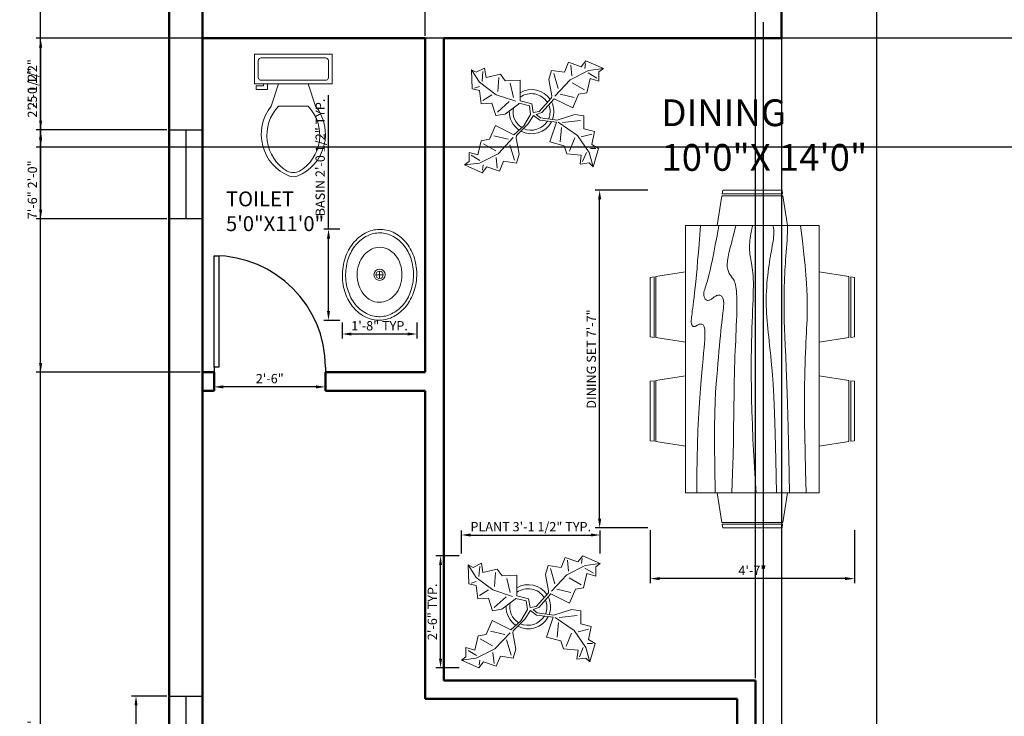
# Model space of a CAD drawing. Units: inches. Extents: x 25547 to 25983, y 30413 to 31159.
# Tile 3 of 5: x 25547 to 25813, y 30790 to 30978. Entities that reach past the tile are written whole.
import ezdxf

# ---------------------------------------------------------------- set-up
doc = ezdxf.new("R2010")
doc.units = ezdxf.units.IN
for name, color, linetype, lineweight in [('A-AREA-IDEN', 11, 'Continuous', 25), ('A-FLOR-FIXT', 6, 'Continuous', 18), ('A-WALL', 7, 'Continuous', 50), ('DIM', 4, 'Continuous', 18), ('DOOR', 3, 'Continuous', 25), ('FLOWER', 60, 'Continuous', 13), ('FURNITURES', 6, 'Continuous', 18), ('WINDOW', 1, 'Continuous', 25)]:
    doc.layers.add(name, color=color, linetype=linetype, lineweight=lineweight)
doc.styles.get("Standard").update_dxf_attribs({"font": 'arial.ttf'})
doc.dimstyles.new('ISO-25', dxfattribs={"dimtxt": 2.5, "dimasz": 2.5, "dimexe": 1.25, "dimexo": 0.625, "dimtad": 1, "dimlunit": 3, "dimtxsty": 'Standard', "dimcen": 2.5, "dimadec": 0, "dimazin": 0, "dimtfac": 1, "dimtmove": 0, "dimatfit": 3, "dimfxl": 1, "dimarcsym": 0})

# ---------------------------------------------------------------- blocks, each defined once
blk = doc.blocks.new('*U5')
for p, q in [((0, 0), (0, -6)), ((40, 0), (40, -6))]:
    blk.add_line(p, q)
blk.add_lwpolyline([(0, 0), (0, 40), (1.75, 40), (1.75, 0)], close=True)
blk.add_arc((0, 0), 40, 0, 90)
blk = doc.blocks.new('Sink - Oval top')
for p, q in [((-1, 0), (1, 0)), ((0, 1), (0, -1))]:
    blk.add_line(p, q)
for points in [[(-12.23, 0.39, 0.117634), (-11.46, -3.36, 0.104469), (-8.88, -6.8, 0.090016), (-5.08, -9.07, 0.08192), (-0.32, -10.02, 0.08192), (4.49, -9.38, 0.090016), (8.42, -7.36, 0.104469), (11.22, -4.09, 0.117634), (12.23, -0.39, 0.117634), (11.46, 3.36, 0.104469), (8.88, 6.8, 0.090016), (5.08, 9.07, 0.08192), (0.32, 10.02, 0.08192), (-4.49, 9.38, 0.090016), (-8.42, 7.36, 0.104469), (-11.22, 4.09, 0.117634)], [(-11.29, 0.16, 0.118622), (-10.52, -3.25, 0.104678), (-8.07, -6.36, 0.089562), (-4.54, -8.37, 0.081185), (-0.13, -9.15, 0.081185), (4.3, -8.49, 0.089562), (7.89, -6.58, 0.104678), (10.42, -3.55, 0.118622), (11.29, -0.16, 0.118622), (10.52, 3.25, 0.104678), (8.07, 6.36, 0.089562), (4.54, 8.37, 0.081185), (0.13, 9.15, 0.081185), (-4.3, 8.49, 0.089562), (-7.89, 6.58, 0.104678), (-10.42, 3.55, 0.118622)], [(-7.42, 0.08, 0.118283), (-6.91, -2.17, 0.104607), (-5.29, -4.21, 0.089718), (-2.97, -5.53, 0.081436), (-0.07, -6.04, 0.081436), (2.84, -5.59, 0.089718), (5.2, -4.33, 0.104607), (6.86, -2.32, 0.118283), (7.42, -0.08, 0.118283), (6.91, 2.17, 0.104607), (5.29, 4.21, 0.089718), (2.97, 5.53, 0.081436), (0.07, 6.04, 0.081436), (-2.84, 5.59, 0.089718), (-5.2, 4.33, 0.104607), (-6.86, 2.32, 0.118283)]]:
    blk.add_lwpolyline(points, format="xyb", close=True)
for radius in [1.5, 1]:
    blk.add_circle((0, 0), radius)
blk = doc.blocks.new('Dining Set - 36 x 72 in.')
for p, q in [((-22, 27.5), (-22.1562, 26.50042)), ((-22, 27.5), (-6, 27.5)), ((-5.8437, 26.49966), (-6, 27.5)), ((6, 27.5), (5.8438, 26.50042)), ((6, 27.5), (22, 27.5)), ((22.1563, 26.49966), (22, 27.5)), ((-22.2343, 26.00059), (-23.4847, 17.99762)), ((-22.2304, 26), (-5.7608, 26)), ((-5.8416, 26.5), (-22.1534, 26.5)), ((-4.5152, 17.99762), (-5.7655, 25.99926)), ((5.7657, 26.00059), (4.5153, 17.99762)), ((5.7696, 26), (22.2392, 26)), ((22.1584, 26.5), (5.8466, 26.5)), ((23.4848, 17.99762), (22.2345, 25.99926)), ((36, 18), (-36, 18)), ((-36, 18), (-36, -18)), ((36, -18), (36, 18)), ((-45.5, 8), (-44.5004, 8.15617)), ((-45.5, 8), (-45.5, -8)), ((-44.5, -8.15843), (-44.5, 8.15338)), ((-44.0006, 8.23428), (-35.9976, 9.48474)), ((-44, 8.23041), (-44, -8.23915)), ((44.0006, 8.23428), (35.9976, 9.48474)), ((44, 8.23041), (44, -8.23915)), ((44.5, -8.15843), (44.5, 8.15338)), ((45.5, 8), (44.5005, 8.15617)), ((45.5, 8), (45.5, -8)), ((-44.4997, -8.15631), (-45.5, -8)), ((-35.9976, -9.48476), (-43.9993, -8.2345)), ((35.9976, -9.48476), (43.9993, -8.2345)), ((44.4997, -8.15631), (45.5, -8)), ((-36, -18), (36, -18)), ((-22.2343, -26.0006), (-23.4847, -17.99762)), ((-4.5152, -17.99762), (-5.7655, -25.99928)), ((5.7657, -26.0006), (4.5153, -17.99762)), ((23.4848, -17.99762), (22.2345, -25.99928)), ((-22.2304, -26), (-5.7608, -26)), ((-22, -27.5), (-22.1562, -26.50044)), ((-5.8416, -26.5), (-22.1534, -26.5)), ((-5.8437, -26.49967), (-6, -27.5)), ((5.7696, -26), (22.2392, -26)), ((6, -27.5), (5.8438, -26.50044)), ((22.1584, -26.5), (5.8466, -26.5)), ((22.1563, -26.49967), (22, -27.5)), ((-22, -27.5), (-6, -27.5)), ((6, -27.5), (22, -27.5))]:
    blk.add_line(p, q)
for points in [[(-36, 15), (-31.1772, 14.97754), (-26.8079, 14.91406), (-22.8538, 14.81543), (-19.276, 14.6875), (-16.0362, 14.53613), (-13.0957, 14.36718), (-10.4159, 14.18652), (-7.9583, 14), (-5.6904, 13.81315), (-3.6035, 13.63021), (-1.6954, 13.45508), (0.0365, 13.29166), (1.5945, 13.14388), (2.9811, 13.01562), (4.1988, 12.9108), (5.25, 12.83333), (6.1393, 12.78613), (6.8802, 12.76823), (7.4883, 12.77767), (7.9792, 12.8125), (8.3685, 12.87077), (8.6719, 12.95052), (8.9049, 13.0498), (9.0833, 13.16666), (9.2205, 13.29899), (9.3216, 13.44401), (9.3895, 13.59879), (9.4271, 13.76041), (9.4373, 13.92594), (9.4232, 14.09245), (9.3875, 14.257), (9.3333, 14.41666), (9.2638, 14.56917), (9.1836, 14.71484), (9.0975, 14.85465), (9.0104, 14.98958), (8.9272, 15.1206), (8.8529, 15.2487), (8.7922, 15.37483), (8.75, 15.5), (8.7305, 15.62467), (8.7344, 15.74739), (8.7617, 15.86621), (8.8125, 15.97916), (8.8867, 16.08431), (8.9844, 16.17968), (9.1055, 16.26334), (9.25, 16.33333), (9.4189, 16.38802), (9.6172, 16.42708), (9.8506, 16.45052), (10.125, 16.45833), (10.4463, 16.45052), (10.8203, 16.42708), (11.2529, 16.38802), (11.75, 16.33333), (12.3184, 16.26318), (12.9694, 16.17838), (13.7151, 16.07991), (14.5677, 15.96875), (15.5395, 15.84586), (16.6426, 15.71224), (17.8893, 15.56884), (19.2917, 15.41666), (20.859, 15.25667), (22.5879, 15.08984), (24.4721, 14.91715), (26.5052, 14.73958), (28.6809, 14.5581), (30.9929, 14.3737), (33.4347, 14.18733), (36, 14)], [(-36, 10), (-28.9766, 10.14274), (-23.1725, 10.20442), (-18.4241, 10.19775), (-14.5677, 10.13541), (-11.4399, 10.03011), (-8.877, 9.89453), (-6.7154, 9.74137), (-4.7917, 9.58333), (-2.9698, 9.43082), (-1.2246, 9.28515), (0.4415, 9.14534), (2.026, 9.01041), (3.5266, 8.87939), (4.9408, 8.7513), (6.266, 8.62516), (7.5, 8.5), (8.6411, 8.37549), (9.6914, 8.2539), (10.6538, 8.13818), (11.5312, 8.03125), (12.3267, 7.93603), (13.043, 7.85547), (13.6831, 7.79248), (14.25, 7.75), (14.7471, 7.7303), (15.1797, 7.73307), (15.5537, 7.75732), (15.875, 7.80208), (16.1494, 7.86637), (16.3828, 7.94922), (16.5811, 8.04964), (16.75, 8.16666), (16.8944, 8.29915), (17.0143, 8.44531), (17.1089, 8.60319), (17.1771, 8.77083), (17.218, 8.94629), (17.2305, 9.1276), (17.2137, 9.31282), (17.1667, 9.5), (17.0895, 9.6875), (16.987, 9.875), (16.8649, 10.0625), (16.7292, 10.25), (16.5856, 10.4375), (16.4401, 10.625), (16.2985, 10.8125), (16.1667, 11), (16.05, 11.18733), (15.9518, 11.3737), (15.8752, 11.5581), (15.8229, 11.73958), (15.798, 11.91715), (15.8034, 12.08984), (15.842, 12.25667), (15.9167, 12.41666), (16.0295, 12.56836), (16.1784, 12.70833), (16.3605, 12.83268), (16.5729, 12.9375), (16.8127, 13.01888), (17.0768, 13.07291), (17.3625, 13.0957), (17.6667, 13.08333), (17.9894, 13.03312), (18.3418, 12.94726), (18.7382, 12.82918), (19.1927, 12.68229), (19.7195, 12.51001), (20.3327, 12.31575), (21.0465, 12.10294), (21.875, 11.875), (22.8357, 11.63354), (23.959, 11.37304), (25.2786, 11.08618), (26.8282, 10.76562), (28.6414, 10.40405), (30.752, 9.99414), (33.1936, 9.52856), (36, 9)], [(-36, 5.5), (-30.7157, 5.3348), (-26.069, 5.20963), (-21.9946, 5.11767), (-18.4271, 5.05208), (-15.3009, 5.00602), (-12.5508, 4.97265), (-10.1112, 4.94515), (-7.9167, 4.91666), (-5.909, 4.88167), (-4.0586, 4.83984), (-2.3429, 4.79215), (-0.7396, 4.73958), (0.7739, 4.6831), (2.22, 4.6237), (3.6213, 4.56233), (5, 4.5), (6.373, 4.43782), (7.7344, 4.3776), (9.0723, 4.32129), (10.375, 4.27083), (11.6309, 4.22819), (12.8281, 4.19531), (13.9551, 4.17415), (15, 4.16666), (15.954, 4.17448), (16.819, 4.19791), (17.6001, 4.23698), (18.3021, 4.29166), (18.9299, 4.36198), (19.4883, 4.44791), (19.9823, 4.54948), (20.4167, 4.66666), (20.7969, 4.79899), (21.1302, 4.94401), (21.4245, 5.09879), (21.6875, 5.26041), (21.9271, 5.42594), (22.1511, 5.59245), (22.3672, 5.757), (22.5834, 5.91666), (22.8065, 6.06868), (23.0404, 6.21093), (23.2879, 6.34147), (23.5521, 6.45833), (23.8358, 6.55957), (24.142, 6.64323), (24.4735, 6.70735), (24.8334, 6.75), (25.2235, 6.76969), (25.642, 6.76692), (26.0858, 6.74267), (26.5521, 6.69791), (27.0379, 6.63362), (27.5404, 6.55078), (28.0565, 6.45036), (28.5834, 6.33333), (29.1242, 6.19987), (29.7071, 6.04687), (30.3661, 5.87044), (31.1354, 5.66666), (32.0493, 5.43164), (33.142, 5.16146), (34.4475, 4.85221), (36, 4.5)], [(-36, -1), (-30.7915, -0.6591), (-26.0195, -0.38216), (-21.6519, -0.16284), (-17.6563, 0.00521), (-14.0005, 0.12833), (-10.6523, 0.21289), (-7.5796, 0.26522), (-4.75, 0.29166), (-2.134, 0.29793), (0.2878, 0.28711), (2.5317, 0.26163), (4.6146, 0.22396), (6.5529, 0.17651), (8.3633, 0.12174), (10.0623, 0.06209), (11.6667, 0), (13.1899, -0.06201), (14.6341, -0.1211), (15.9982, -0.17432), (17.2813, -0.21875), (18.4823, -0.25147), (19.6003, -0.26953), (20.6343, -0.27002), (21.5834, -0.25), (22.4481, -0.20768), (23.2357, -0.14584), (23.9549, -0.06836), (24.6146, 0.02083), (25.2235, 0.11784), (25.7904, 0.21875), (26.3241, 0.31966), (26.8334, 0.41666), (27.3265, 0.50618), (27.8099, 0.58593), (28.2894, 0.65397), (28.7709, 0.70833), (29.2601, 0.74707), (29.763, 0.76823), (30.2855, 0.76985), (30.8334, 0.75), (31.4088, 0.70784), (31.9994, 0.64713), (32.589, 0.57275), (33.1615, 0.48958), (33.7008, 0.4025), (34.1908, 0.3164), (34.6153, 0.23616), (34.9584, 0.16666), (35.2099, 0.11165), (35.3848, 0.07031), (35.504, 0.04069), (35.5886, 0.02083), (35.6594, 0.00879), (35.7377, 0.0026), (35.8442, 0.00032), (36, 0)], [(-36, -6.5), (-27.1843, -6.31267), (-20.084, -6.1263), (-14.469, -5.9419), (-10.1094, -5.76042), (-6.7752, -5.58285), (-4.2363, -5.41016), (-2.2629, -5.24333), (-0.625, -5.08334), (0.8708, -4.93099), (2.2715, -4.78646), (3.5872, -4.64974), (4.8281, -4.52084), (6.0046, -4.39974), (7.127, -4.28646), (8.2053, -4.18099), (9.25, -4.08334), (10.2705, -3.99382), (11.2734, -3.91407), (12.2647, -3.84603), (13.25, -3.79167), (14.2354, -3.75293), (15.2266, -3.73177), (16.2295, -3.73015), (17.25, -3.75), (18.2912, -3.79248), (19.3451, -3.85547), (20.4009, -3.93604), (21.4479, -4.03125), (22.4754, -4.13819), (23.4727, -4.25391), (24.4289, -4.37549), (25.3334, -4.5), (26.1785, -4.62492), (26.9694, -4.74935), (27.7145, -4.87281), (28.4219, -4.99479), (29.1, -5.11483), (29.7572, -5.23242), (30.4016, -5.34709), (31.0417, -5.45834), (31.6837, -5.56437), (32.3262, -5.65821), (32.9658, -5.73153), (33.599, -5.77604), (34.2224, -5.78345), (34.8327, -5.74545), (35.4264, -5.65373), (36, -5.5)], [(-36, -10), (-26.4022, -9.81299), (-18.4675, -9.62891), (-11.9839, -9.45069), (-6.7396, -9.28125), (-2.5226, -9.12354), (0.8789, -8.98047), (3.6769, -8.85498), (6.0833, -8.75), (8.2767, -8.66765), (10.3021, -8.60677), (12.1712, -8.56543), (13.8958, -8.54167), (15.4876, -8.53353), (16.9583, -8.53907), (18.3197, -8.55632), (19.5834, -8.58334), (20.7616, -8.61841), (21.8685, -8.66081), (22.9188, -8.71004), (23.9271, -8.76563), (24.9081, -8.82707), (25.8763, -8.89388), (26.8465, -8.96558), (27.8334, -9.04167), (28.8474, -9.12118), (29.8828, -9.20117), (30.93, -9.27824), (31.9792, -9.34896), (33.0205, -9.40991), (34.0443, -9.45768), (35.0407, -9.48885), (36, -9.5)], [(-36, -14.5), (-30.0881, -14.33513), (-25.0332, -14.21224), (-20.7312, -14.12647), (-17.0781, -14.07292), (-13.97, -14.04671), (-11.3027, -14.04297), (-8.9724, -14.05681), (-6.875, -14.08334), (-4.9224, -14.11833), (-3.0905, -14.16016), (-1.3709, -14.20785), (0.2448, -14.26042), (1.7647, -14.3169), (3.1973, -14.3763), (4.5507, -14.43767), (5.8333, -14.5), (7.0554, -14.5621), (8.235, -14.62175), (9.3922, -14.67652), (10.5469, -14.72396), (11.7192, -14.76164), (12.929, -14.78711), (14.1965, -14.79794), (15.5417, -14.79167), (16.9933, -14.76424), (18.6152, -14.70508), (20.4804, -14.60197), (22.6615, -14.44271), (25.2312, -14.21509), (28.2624, -13.9069), (31.8277, -13.50594), (36, -13)]]:
    blk.add_lwpolyline(points)
blk = doc.blocks.new('Toilet - top')
for p, q in [((9.5, -6), (9.5, -2)), ((-10, -8.5), (-8, -8.5)), ((-10, -9.5), (-10, -8.5)), ((-7, -9.5), (-10, -9.5)), ((-8, -8.5), (-8, -8)), ((-7, -8), (-7, -9.5)), ((-4, -8), (-6, -14)), ((4, -8), (6, -14)), ((4, -14), (-4, -14))]:
    blk.add_line(p, q)
blk.add_lwpolyline([(10.5, -8), (10.5, 0), (-10.5, 0), (-10.5, -8)], close=True)
for points in [[(-9.5, -2), (-9.5, -6)], [(8.5, -1), (-8.5, -1)], [(-8.5, -7), (8.5, -7)]]:
    blk.add_lwpolyline(points)
for centre, radius, start, end in [((-8.62, -1.88), 0.884, 81.8699, 188.1301), ((8.62, -1.88), 0.884, 351.8699, 98.1301), ((-8.62, -6.12), 0.884, 171.8699, 278.1301), ((8.62, -6.12), 0.884, 261.8699, 8.1301), ((3.52, -21.58), 12.17, 141.4691, 247.9714), ((4.2, -21.82), 11.33, 136.3677, 238.9468), ((-3.52, -21.58), 12.17, 292.0284, 38.5307), ((-4.2, -21.82), 11.33, 301.053, 43.6321), ((0, -27.88), 4, 245.7318, 294.2682), ((0, -29), 4, 254.8605, 285.1395)]:
    blk.add_arc(centre, radius, start, end)
blk = doc.blocks.new('Plant - Rubber or Philodendron')
for p, q in [((8.8871, 10.7908), (9.9809, 13.4933)), ((9.9809, 13.4933), (13.3837, 12.301)), ((13.3837, 12.301), (14.68, 13.9039)), ((14.68, 13.9039), (19.3848, 11.8146)), ((-16.2005, 11.4774), (-13.9899, 8.1064)), ((-16.2005, 11.4774), (-14.8639, 10.7964)), ((-16.0159, 6.3329), (-16.2005, 11.4774)), ((-14.8639, 10.7964), (-12.6195, 11.8975)), ((-13.3174, 8.325), (-13.0735, 11.0065)), ((-12.6195, 11.8975), (-12.1909, 9.4345)), ((4.6914, 8.8812), (5.3859, 11.2828)), ((5.3859, 11.2828), (8.8871, 10.7908)), ((15.3859, 11.3055), (10.3916, 8.7942)), ((10.5828, 12.6946), (10.8893, 9.7953)), ((14.5816, 13.2037), (14.3848, 11.8033)), ((19.3848, 11.8146), (15.3859, 11.3055)), ((19.3848, 11.8146), (18.1868, 10.9119)), ((18.1868, 10.9119), (18.1925, 8.4119)), ((-13.9899, 8.1064), (-9.5434, 4.7185)), ((-12.1909, 9.4345), (-8.3829, 10.3)), ((-8.8369, 9.409), (-9.0894, 5.6095)), ((-8.3829, 10.3), (-7.0549, 8.501)), ((-7.0549, 8.501), (-3.0284, 8.6941)), ((-3.0284, 8.6941), (-3.0709, 3.1041)), ((4.6914, 8.8812), (5.5014, 4.4831)), ((5.9878, 10.4842), (7.1971, 6.3869)), ((10.3916, 8.7942), (6.2847, 4.4028)), ((14.2977, 6.1031), (10.9934, 7.9956)), ((15.7909, 9.1065), (14.8995, 5.3044)), ((15.2875, 10.6053), (17.5907, 9.2105)), ((18.1925, 8.4119), (15.7909, 9.1065)), ((-14.0069, 5.8704), (-16.0159, 6.3329)), ((-15.3434, 6.5514), (-13.9984, 6.9884)), ((-13.5868, 2.2894), (-14.0069, 5.8704)), ((-4.8529, 4.012), (-5.7184, 7.82)), ((-13.1329, 3.1804), (-10.6614, 4.727)), ((-9.5434, 4.7185), (-4.1917, 2.9888)), ((-9.1318, 0.0195), (-5.9793, 2.9025)), ((-3.0709, 3.1041), (0.0797, 2.3163)), ((2.1141, 0.2298), (5.4346, 3.9146)), ((6.1032, 3.6844), (2.8262, -0.031)), ((5.4346, 3.9146), (5.5014, 4.4831)), ((11.1089, 1.1958), (6.1032, 3.6844)), ((7.7005, 4.8881), (11.5025, 3.9967)), ((12.7005, 4.8994), (11.1089, 1.1958)), ((14.8995, 5.3044), (12.7005, 4.8994)), ((-10.6784, 2.491), (-13.5868, 2.2894)), ((-9.5858, -0.8715), (-10.6784, 2.491)), ((-7.1228, -0.443), (-3.5248, 2.2131)), ((-3.5248, 2.2131), (-3.3011, 2.4355)), ((-3.3011, 2.4355), (-0.5306, 1.7947)), ((-0.5306, 1.7947), (-0.2255, -0.5527)), ((-0.5306, 1.7947), (-0.5306, 1.7947)), ((0.0797, 2.3163), (0.4866, -0.031)), ((0.4866, -0.031), (2.1141, 0.2298)), ((-7.1228, -0.443), (-9.5858, -0.8715)), ((-2.019, -3.6148), (-0.2255, -0.5527)), ((-0.9375, -3.1608), (0.5883, -0.8135)), ((0.5883, -0.8135), (2.2447, -2.0916)), ((2.8262, -0.031), (1.3003, -0.5527)), ((1.3003, -0.5527), (2.4193, -1.4655)), ((2.2447, -2.0916), (6.7108, -2.6626)), ((2.4193, -1.4655), (6.895, -2.1175)), ((11.6605, -0.5413), (6.895, -2.1175)), ((8.3544, -2.7453), (13.1973, -2.1704)), ((11.6605, -0.5413), (14.1354, -0.8948)), ((14.1354, -0.8948), (14.1354, -4.4304)), ((-11.3237, -7.2629), (-9.7321, -3.5593)), ((-9.7321, -3.5593), (-4.7264, -6.0479)), ((-2.019, -3.6148), (-4.7264, -6.0479)), ((-4.0579, -6.2781), (-0.9375, -3.1608)), ((4.943, -7.9659), (6.7108, -2.6626)), ((12.3677, -6.1981), (7.219, -2.6772)), ((8.125, -4.0768), (7.7715, -7.9659)), ((14.1354, -4.4304), (16.9638, -5.1375)), ((16.9638, -5.1375), (16.2567, -8.673)), ((-14.4141, -11.4699), (-13.5228, -7.6679)), ((-13.5228, -7.6679), (-11.3237, -7.2629)), ((-6.3237, -7.2516), (-10.1257, -6.3602)), ((-9.0148, -11.1577), (-4.9047, -6.8122)), ((-4.1246, -6.8466), (-4.0579, -6.2781)), ((-3.3146, -11.2447), (-4.1246, -6.8466)), ((10.2463, -10.4408), (11.6605, -6.9053)), ((15.5496, -10.7943), (12.3677, -6.1981)), ((16.2567, -5.8446), (13.4283, -6.5517)), ((-12.921, -8.4665), (-9.6166, -10.359)), ((-4.611, -12.8477), (-5.8203, -8.7504)), ((8.8321, -9.0266), (4.943, -7.9659)), ((9.5392, -11.1479), (8.8321, -9.0266)), ((17.3174, -9.7337), (15.9032, -9.7337)), ((16.2567, -8.673), (18.0245, -9.7337)), ((18.0245, -9.7337), (16.6103, -14.6834)), ((-16.8157, -10.7754), (-14.4141, -11.4699)), ((-16.8101, -13.2754), (-16.8157, -10.7754)), ((-13.9107, -12.9688), (-16.2139, -11.574)), ((-14.0091, -13.669), (-9.0148, -11.1577)), ((-9.206, -15.0581), (-9.5126, -12.1588)), ((-7.5103, -13.1543), (-8.6042, -15.8568)), ((-4.0092, -13.6463), (-7.5103, -13.1543)), ((-3.3146, -11.2447), (-4.0092, -13.6463)), ((13.4283, -11.5015), (9.5392, -11.1479)), ((13.0748, -13.9763), (13.4283, -11.5015)), ((14.8425, -10.7943), (13.7819, -13.2692)), ((16.6103, -14.6834), (15.5496, -10.7943)), ((-18.008, -14.1781), (-16.8101, -13.2754)), ((-18.008, -14.1781), (-14.0091, -13.669)), ((-13.3032, -16.2674), (-18.008, -14.1781)), ((-12.0069, -14.6645), (-13.3032, -16.2674)), ((-13.2048, -15.5672), (-13.008, -14.1668)), ((-8.6042, -15.8568), (-12.0069, -14.6645)), ((15.5496, -13.6228), (13.0748, -13.9763)), ((16.6103, -14.6834), (15.5496, -13.6228))]:
    blk.add_line(p, q)
for centre, radius, start, end in [((0, 0), 6.1275, 34.37569, 120.1028), ((-0.0601, -0.2075), 5.2461, 33.82192, 124.9414), ((-0.098, 0.1364), 6.1288, 341.2017, 26.09184), ((0.0308, 0.1664), 6, 178.6147, 235.1169), ((0.0308, 0.1664), 5, 168.1647, 238.6725), ((-0.2664, 0.1682), 5.2775, 338.4094, 20.03007), ((-0.0234, 0.3825), 6.1492, 242.5812, 331.2714), ((-0.1102, 0.4886), 5.2883, 247.3711, 327.472)]:
    blk.add_arc(centre, radius, start, end)
blk = doc.blocks.new('*D25')
at = {"layer": 'Defpoints', "color": 0, "transparency": 16777216}
for p in [(25599.62, 30878.91), (25599.62, 30877.83), (25629.62, 30877.83)]:
    blk.add_point(p, dxfattribs=at)
at = {"layer": 'DIM', "color": 0, "lineweight": -2, "transparency": 16777216}
for p, q in [((25599.62, 30878.45), (25599.62, 30880.16)), ((25629.62, 30878.45), (25629.62, 30880.16)), ((25627.12, 30878.91), (25602.12, 30878.91))]:
    blk.add_line(p, q, dxfattribs=at)
at = {"layer": 'DIM', "color": 0, "transparency": 16777216}
for points in [[(25602.12, 30879.32), (25602.12, 30878.49), (25599.62, 30878.91)], [(25627.12, 30879.32), (25627.12, 30878.49), (25629.62, 30878.91)]]:
    blk.add_solid(points, dxfattribs=at)
at = {"layer": 'DIM', "color": 0, "transparency": 16777216, "insert": (25614.62, 30880.81), "char_height": 2.5, "attachment_point": 5}
blk.add_mtext('2\'-6"', dxfattribs=at)
blk = doc.blocks.new('*D26')
at = {"layer": 'Defpoints', "color": 0, "transparency": 16777216}
for p in [(25587.53, 30795.61), (25578.58, 30747.61), (25587.53, 30747.61)]:
    blk.add_point(p, dxfattribs=at)
at = {"layer": 'DIM', "color": 0, "lineweight": -2, "transparency": 16777216}
for p, q in [((25586.9, 30795.61), (25577.33, 30795.61)), ((25578.58, 30793.11), (25578.58, 30750.11)), ((25586.9, 30747.61), (25577.33, 30747.61))]:
    blk.add_line(p, q, dxfattribs=at)
at = {"layer": 'DIM', "color": 0, "transparency": 16777216}
for points in [[(25578.17, 30793.11), (25579, 30793.11), (25578.58, 30795.61)], [(25578.17, 30750.11), (25579, 30750.11), (25578.58, 30747.61)]]:
    blk.add_solid(points, dxfattribs=at)
at = {"layer": 'DIM', "color": 0, "transparency": 16777216, "insert": (25576.71, 30771.61), "char_height": 2.5, "attachment_point": 5, "rotation": 90}
blk.add_mtext("4'", dxfattribs=at)
blk = doc.blocks.new('*D31')
at = {"layer": 'Defpoints', "color": 0, "transparency": 16777216}
for p in [(25656.53, 30981.43), (25596.53, 30972.83), (25656.53, 30972.83)]:
    blk.add_point(p, dxfattribs=at)
at = {"layer": 'DIM', "color": 0, "lineweight": -2, "transparency": 16777216}
for p, q in [((25596.53, 30973.45), (25596.53, 30982.68)), ((25656.53, 30973.45), (25656.53, 30982.68)), ((25599.03, 30981.43), (25654.03, 30981.43))]:
    blk.add_line(p, q, dxfattribs=at)
at = {"layer": 'DIM', "color": 0, "transparency": 16777216}
for points in [[(25599.03, 30981.85), (25599.03, 30981.01), (25596.53, 30981.43)], [(25654.03, 30981.85), (25654.03, 30981.01), (25656.53, 30981.43)]]:
    blk.add_solid(points, dxfattribs=at)
at = {"layer": 'DIM', "color": 0, "transparency": 16777216, "insert": (25626.53, 30983.32), "char_height": 2.5, "attachment_point": 5}
blk.add_mtext("5'", dxfattribs=at)
blk = doc.blocks.new('WIN-48IN')
blk.add_line((4.5, 48), (4.5, 0))
blk.add_lwpolyline([(0, 48), (9, 48), (9, 0), (0, 0)], close=True)
blk = doc.blocks.new('WIN-24IN')
blk.add_line((0, 4.5), (24, 4.5))
blk.add_lwpolyline([(0, 0), (0, 9), (24, 9), (24, 0)], close=True)
blk = doc.blocks.new('*D42')
at = {"layer": 'Defpoints', "color": 0, "transparency": 16777216}
for p in [(25630.45, 30921.38), (25634.13, 30921.38), (25634.13, 30896.83)]:
    blk.add_point(p, dxfattribs=at)
at = {"layer": 'DIM', "color": 0, "lineweight": -2, "transparency": 16777216}
for p, q in [((25630.45, 30921.38), (25630.45, 30957.54)), ((25633.51, 30921.38), (25629.2, 30921.38)), ((25630.45, 30899.33), (25630.45, 30918.88)), ((25633.51, 30896.83), (25629.2, 30896.83))]:
    blk.add_line(p, q, dxfattribs=at)
at = {"layer": 'DIM', "color": 0, "transparency": 16777216}
for points in [[(25630.04, 30918.88), (25630.87, 30918.88), (25630.45, 30921.38)], [(25630.04, 30899.33), (25630.87, 30899.33), (25630.45, 30896.83)]]:
    blk.add_solid(points, dxfattribs=at)
at = {"layer": 'DIM', "color": 0, "transparency": 16777216, "insert": (25628.53, 30940.71), "char_height": 2.5, "attachment_point": 5, "rotation": 90}
blk.add_mtext('BASIN 2\'-0 1/2" TYP.', dxfattribs=at)
blk = doc.blocks.new('*D43')
at = {"layer": 'Defpoints', "color": 0, "transparency": 16777216}
for p in [(25634.13, 30896.83), (25654.27, 30896.83), (25634.13, 30893.15)]:
    blk.add_point(p, dxfattribs=at)
at = {"layer": 'DIM', "color": 0, "lineweight": -2, "transparency": 16777216}
for p, q in [((25634.13, 30896.21), (25634.13, 30891.9)), ((25654.27, 30896.21), (25654.27, 30891.9)), ((25651.77, 30893.15), (25636.63, 30893.15))]:
    blk.add_line(p, q, dxfattribs=at)
at = {"layer": 'DIM', "color": 0, "transparency": 16777216}
for points in [[(25636.63, 30893.56), (25636.63, 30892.73), (25634.13, 30893.15)], [(25651.77, 30893.56), (25651.77, 30892.73), (25654.27, 30893.15)]]:
    blk.add_solid(points, dxfattribs=at)
at = {"layer": 'DIM', "color": 0, "transparency": 16777216, "insert": (25644.2, 30895.05), "char_height": 2.5, "attachment_point": 5}
blk.add_mtext('1\'-8" TYP.', dxfattribs=at)
blk = doc.blocks.new('*D46')
at = {"layer": 'Defpoints', "color": 0, "transparency": 16777216}
for p in [(25703.64, 30839), (25666.25, 30833.39), (25703.64, 30833.39)]:
    blk.add_point(p, dxfattribs=at)
at = {"layer": 'DIM', "color": 0, "lineweight": -2, "transparency": 16777216}
for p, q in [((25666.25, 30834.02), (25666.25, 30840.25)), ((25703.64, 30834.02), (25703.64, 30840.25)), ((25668.75, 30839), (25701.14, 30839))]:
    blk.add_line(p, q, dxfattribs=at)
at = {"layer": 'DIM', "color": 0, "transparency": 16777216}
for points in [[(25668.75, 30839.42), (25668.75, 30838.59), (25666.25, 30839)], [(25701.14, 30839.42), (25701.14, 30838.59), (25703.64, 30839)]]:
    blk.add_solid(points, dxfattribs=at)
at = {"layer": 'DIM', "color": 0, "transparency": 16777216, "insert": (25684.94, 30840.92), "char_height": 2.5, "attachment_point": 5}
blk.add_mtext('PLANT 3\'-1 1/2" TYP.', dxfattribs=at)
blk = doc.blocks.new('*D47')
at = {"layer": 'Defpoints', "color": 0, "transparency": 16777216}
for p in [(25660.64, 30833.39), (25666.25, 30833.39), (25666.25, 30803.22)]:
    blk.add_point(p, dxfattribs=at)
at = {"layer": 'DIM', "color": 0, "lineweight": -2, "transparency": 16777216}
for p, q in [((25665.62, 30833.39), (25659.39, 30833.39)), ((25660.64, 30805.72), (25660.64, 30830.89)), ((25665.62, 30803.22), (25659.39, 30803.22))]:
    blk.add_line(p, q, dxfattribs=at)
at = {"layer": 'DIM', "color": 0, "transparency": 16777216}
for points in [[(25660.22, 30830.89), (25661.05, 30830.89), (25660.64, 30833.39)], [(25660.22, 30805.72), (25661.05, 30805.72), (25660.64, 30803.22)]]:
    blk.add_solid(points, dxfattribs=at)
at = {"layer": 'DIM', "color": 0, "transparency": 16777216, "insert": (25658.74, 30818.31), "char_height": 2.5, "attachment_point": 5, "rotation": 90}
blk.add_mtext('2\'-6" TYP.', dxfattribs=at)
blk = doc.blocks.new('*D60')
at = {"layer": 'Defpoints', "color": 0, "transparency": 16777216}
for p in [(25703.5, 30931.9), (25717.15, 30931.9), (25717.15, 30840.9)]:
    blk.add_point(p, dxfattribs=at)
at = {"layer": 'DIM', "color": 0, "lineweight": -2, "transparency": 16777216}
for p, q in [((25716.52, 30931.9), (25702.25, 30931.9)), ((25703.5, 30843.4), (25703.5, 30929.4)), ((25716.52, 30840.9), (25702.25, 30840.9))]:
    blk.add_line(p, q, dxfattribs=at)
at = {"layer": 'DIM', "color": 0, "transparency": 16777216}
for points in [[(25703.08, 30929.4), (25703.92, 30929.4), (25703.5, 30931.9)], [(25703.08, 30843.4), (25703.92, 30843.4), (25703.5, 30840.9)]]:
    blk.add_solid(points, dxfattribs=at)
at = {"layer": 'DIM', "color": 0, "transparency": 16777216, "insert": (25701.58, 30886.4), "char_height": 2.5, "attachment_point": 5, "rotation": 90}
blk.add_mtext('DINING SET 7\'-7"', dxfattribs=at)
blk = doc.blocks.new('*D61')
at = {"layer": 'Defpoints', "color": 0, "transparency": 16777216}
for p in [(25717.15, 30840.9), (25772.15, 30840.9), (25717.15, 30827.25)]:
    blk.add_point(p, dxfattribs=at)
at = {"layer": 'DIM', "color": 0, "lineweight": -2, "transparency": 16777216}
for p, q in [((25717.15, 30840.28), (25717.15, 30826)), ((25772.15, 30840.28), (25772.15, 30826)), ((25769.65, 30827.25), (25719.65, 30827.25))]:
    blk.add_line(p, q, dxfattribs=at)
at = {"layer": 'DIM', "color": 0, "transparency": 16777216}
for points in [[(25719.65, 30827.67), (25719.65, 30826.84), (25717.15, 30827.25)], [(25769.65, 30827.67), (25769.65, 30826.84), (25772.15, 30827.25)]]:
    blk.add_solid(points, dxfattribs=at)
at = {"layer": 'DIM', "color": 0, "transparency": 16777216, "insert": (25744.65, 30829.13), "char_height": 2.5, "attachment_point": 5}
blk.add_mtext('4\'-7"', dxfattribs=at)
blk = doc.blocks.new('*D68')
at = {"layer": 'Defpoints', "color": 0, "transparency": 16777216}
for p in [(25552.89, 31118.83), (25587.53, 31118.83), (25587.53, 30449.83)]:
    blk.add_point(p, dxfattribs=at)
at = {"layer": 'DIM', "color": 0, "lineweight": -2, "transparency": 16777216}
for p, q in [((25586.9, 31118.83), (25551.64, 31118.83)), ((25552.89, 30452.33), (25552.89, 31116.33)), ((25586.9, 30449.83), (25551.64, 30449.83))]:
    blk.add_line(p, q, dxfattribs=at)
at = {"layer": 'DIM', "color": 0, "transparency": 16777216}
for points in [[(25552.47, 31116.33), (25553.31, 31116.33), (25552.89, 31118.83)], [(25552.47, 30452.33), (25553.31, 30452.33), (25552.89, 30449.83)]]:
    blk.add_solid(points, dxfattribs=at)
at = {"layer": 'DIM', "color": 0, "transparency": 16777216, "insert": (25550.99, 30784.33), "char_height": 2.5, "attachment_point": 5, "rotation": 90}
blk.add_mtext('55\'-9"', dxfattribs=at)
blk = doc.blocks.new('*D77')
at = {"layer": 'Defpoints', "color": 0, "transparency": 16777216}
for p in [(25596.53, 30977.83), (25747.53, 30977.83), (25747.53, 30415.19)]:
    blk.add_point(p, dxfattribs=at)
at = {"layer": 'DIM', "color": 0, "lineweight": -2, "transparency": 16777216}
for p, q in [((25596.53, 30977.2), (25596.53, 30413.94)), ((25747.53, 30977.2), (25747.53, 30413.94)), ((25599.03, 30415.19), (25745.03, 30415.19))]:
    blk.add_line(p, q, dxfattribs=at)
at = {"layer": 'DIM', "color": 0, "transparency": 16777216}
for points in [[(25599.03, 30415.61), (25599.03, 30414.77), (25596.53, 30415.19)], [(25745.03, 30415.61), (25745.03, 30414.77), (25747.53, 30415.19)]]:
    blk.add_solid(points, dxfattribs=at)
at = {"layer": 'DIM', "color": 0, "transparency": 16777216, "insert": (25672.03, 30417.07), "char_height": 2.5, "attachment_point": 5}
blk.add_mtext('12\'-7"', dxfattribs=at)
blk = doc.blocks.new('*D80')
at = {"layer": 'Defpoints', "color": 0, "transparency": 16777216}
for p in [(25552.89, 30972.83), (25596.53, 30972.83), (25596.53, 30882.83)]:
    blk.add_point(p, dxfattribs=at)
at = {"layer": 'DIM', "color": 0, "lineweight": -2, "transparency": 16777216}
for p, q in [((25595.9, 30972.83), (25551.64, 30972.83)), ((25552.89, 30885.33), (25552.89, 30970.33)), ((25595.9, 30882.83), (25551.64, 30882.83))]:
    blk.add_line(p, q, dxfattribs=at)
at = {"layer": 'DIM', "color": 0, "transparency": 16777216}
for points in [[(25552.47, 30970.33), (25553.31, 30970.33), (25552.89, 30972.83)], [(25552.47, 30885.33), (25553.31, 30885.33), (25552.89, 30882.83)]]:
    blk.add_solid(points, dxfattribs=at)
at = {"layer": 'DIM', "color": 0, "transparency": 16777216, "insert": (25550.99, 30927.83), "char_height": 2.5, "attachment_point": 5, "rotation": 90}
blk.add_mtext('7\'-6"', dxfattribs=at)
blk = doc.blocks.new('*D81')
at = {"layer": 'Defpoints', "color": 0, "transparency": 16777216}
for p in [(25587.53, 30948.15), (25552.89, 30924.15), (25587.53, 30924.15)]:
    blk.add_point(p, dxfattribs=at)
at = {"layer": 'DIM', "color": 0, "lineweight": -2, "transparency": 16777216}
for p, q in [((25586.9, 30948.15), (25551.64, 30948.15)), ((25552.89, 30945.65), (25552.89, 30926.65)), ((25586.9, 30924.15), (25551.64, 30924.15))]:
    blk.add_line(p, q, dxfattribs=at)
at = {"layer": 'DIM', "color": 0, "transparency": 16777216}
for points in [[(25552.47, 30945.65), (25553.31, 30945.65), (25552.89, 30948.15)], [(25552.47, 30926.65), (25553.31, 30926.65), (25552.89, 30924.15)]]:
    blk.add_solid(points, dxfattribs=at)
at = {"layer": 'DIM', "color": 0, "transparency": 16777216, "insert": (25550.99, 30936.15), "char_height": 2.5, "attachment_point": 5, "rotation": 90}
blk.add_mtext('2\'-0"', dxfattribs=at)
blk = doc.blocks.new('*D82')
at = {"layer": 'Defpoints', "color": 0, "transparency": 16777216}
for p in [(25552.89, 30972.83), (25596.53, 30972.83), (25587.53, 30948.15)]:
    blk.add_point(p, dxfattribs=at)
at = {"layer": 'DIM', "color": 0, "lineweight": -2, "transparency": 16777216}
for p, q in [((25595.9, 30972.83), (25551.64, 30972.83)), ((25552.89, 30950.65), (25552.89, 30970.33)), ((25586.9, 30948.15), (25551.64, 30948.15))]:
    blk.add_line(p, q, dxfattribs=at)
at = {"layer": 'DIM', "color": 0, "transparency": 16777216}
for points in [[(25552.47, 30970.33), (25553.31, 30970.33), (25552.89, 30972.83)], [(25552.47, 30950.65), (25553.31, 30950.65), (25552.89, 30948.15)]]:
    blk.add_solid(points, dxfattribs=at)
at = {"layer": 'DIM', "color": 0, "transparency": 16777216, "insert": (25550.97, 30960.49), "char_height": 2.5, "attachment_point": 5, "rotation": 90}
blk.add_mtext('2\'-0 1/2"', dxfattribs=at)
blk = doc.blocks.new('*D92')
at = {"layer": 'Defpoints', "color": 0, "transparency": 16777216}
for p in [(25848.01, 30972.83), (25552.89, 30943.48), (25848.01, 30943.48)]:
    blk.add_point(p, dxfattribs=at)
at = {"layer": 'DIM', "color": 0, "lineweight": -2, "transparency": 16777216}
for p, q in [((25847.38, 30972.83), (25551.64, 30972.83)), ((25552.89, 30970.33), (25552.89, 30945.98)), ((25847.38, 30943.48), (25551.64, 30943.48))]:
    blk.add_line(p, q, dxfattribs=at)
at = {"layer": 'DIM', "color": 0, "transparency": 16777216}
for points in [[(25552.47, 30970.33), (25553.31, 30970.33), (25552.89, 30972.83)], [(25552.47, 30945.98), (25553.31, 30945.98), (25552.89, 30943.48)]]:
    blk.add_solid(points, dxfattribs=at)
at = {"layer": 'DIM', "color": 0, "transparency": 16777216, "insert": (25550.97, 30958.15), "char_height": 2.5, "attachment_point": 5, "rotation": 90}
blk.add_mtext('2\'-5 1/2"', dxfattribs=at)
blk = doc.blocks.new('*D99')
at = {"layer": 'Defpoints', "color": 0, "transparency": 16777216}
for p in [(25836.53, 31153.47), (25745.53, 30799.83), (25836.53, 30794.83)]:
    blk.add_point(p, dxfattribs=at)
at = {"layer": 'DIM', "color": 0, "lineweight": -2, "transparency": 16777216}
for p, q in [((25745.53, 30800.45), (25745.53, 31154.72)), ((25748.03, 31153.47), (25834.03, 31153.47)), ((25836.53, 30795.45), (25836.53, 31154.72))]:
    blk.add_line(p, q, dxfattribs=at)
at = {"layer": 'DIM', "color": 0, "transparency": 16777216}
for points in [[(25748.03, 31153.88), (25748.03, 31153.05), (25745.53, 31153.47)], [(25834.03, 31153.88), (25834.03, 31153.05), (25836.53, 31153.47)]]:
    blk.add_solid(points, dxfattribs=at)
at = {"layer": 'DIM', "color": 0, "transparency": 16777216, "insert": (25791.03, 31155.34), "char_height": 2.5, "attachment_point": 5}
blk.add_mtext('7\'-7"', dxfattribs=at)
blk = doc.blocks.new('*D103')
at = {"layer": 'Defpoints', "color": 0, "transparency": 16777216}
for p in [(25752.53, 31019.83), (25778.13, 31019.83), (25778.13, 30415.19)]:
    blk.add_point(p, dxfattribs=at)
at = {"layer": 'DIM', "color": 0, "lineweight": -2, "transparency": 16777216}
for p, q in [((25752.53, 31019.2), (25752.53, 30413.94)), ((25778.13, 31019.2), (25778.13, 30413.94)), ((25755.03, 30415.19), (25775.63, 30415.19))]:
    blk.add_line(p, q, dxfattribs=at)
at = {"layer": 'DIM', "color": 0, "transparency": 16777216}
for points in [[(25755.03, 30415.61), (25755.03, 30414.77), (25752.53, 30415.19)], [(25775.63, 30415.61), (25775.63, 30414.77), (25778.13, 30415.19)]]:
    blk.add_solid(points, dxfattribs=at)
at = {"layer": 'DIM', "color": 0, "transparency": 16777216, "insert": (25765.33, 30417.11), "char_height": 2.5, "attachment_point": 5}
blk.add_mtext('2\'-1 1/2"', dxfattribs=at)

msp = doc.modelspace()

# ---------------------------------------------------------------- linework, layer by layer
at = {"layer": 'A-WALL'}
for p, q in [((25587.528, 30852.828), (25587.528, 31118.828)), ((25596.528, 30650.828), (25596.528, 31109.828)), ((25752.528, 30972.828), (25752.528, 30981.569)), ((25596.528, 30972.828), (25656.528, 30972.828)), ((25656.528, 30882.828), (25656.528, 30972.828)), ((25661.528, 30799.828), (25661.528, 30972.828)), ((25661.528, 30972.828), (25745.528, 30972.828)), ((25745.528, 30972.828), (25752.528, 30972.828)), ((25596.528, 30882.828), (25599.617, 30882.828)), ((25629.617, 30882.828), (25656.528, 30882.828)), ((25596.528, 30877.828), (25599.617, 30877.828)), ((25629.617, 30877.828), (25656.528, 30877.828)), ((25656.528, 30794.828), (25656.528, 30877.828)), ((25587.528, 30449.828), (25587.528, 30852.828)), ((25661.528, 30799.828), (25661.528, 30847.828)), ((25661.528, 30799.828), (25745.528, 30799.828)), ((25745.528, 30782.944), (25745.528, 30799.828)), ((25656.528, 30794.828), (25740.528, 30794.828)), ((25740.528, 30782.944), (25740.528, 30794.828))]:
    msp.add_line(p, q, dxfattribs=at)
for points in [[(25599.617, 30877.828), (25599.617, 30882.828)], [(25629.617, 30882.828), (25629.617, 30877.828)]]:
    msp.add_lwpolyline(points, dxfattribs=at)

# ---------------------------------------------------------------- block references
at = {"layer": 'A-FLOR-FIXT'}
msp.add_blockref('Toilet - top', (25620.975, 30968.522), dxfattribs=at)
at = {"layer": 'A-FLOR-FIXT', "rotation": 90}
msp.add_blockref('Sink - Oval top', (25644.203, 30909.106), dxfattribs=at)
at = {"layer": 'DOOR', "xscale": 0.75, "yscale": 0.75, "zscale": 0.75}
msp.add_blockref('*U5', (25599.617, 30884.233), dxfattribs=at)
at = {"layer": 'FLOWER'}
for p in [(25685.134, 30952.864), (25684.254, 30819.489)]:
    msp.add_blockref('Plant - Rubber or Philodendron', p, dxfattribs=at)
at = {"layer": 'FURNITURES', "rotation": 90}
msp.add_blockref('Dining Set - 36 x 72 in.', (25744.649, 30886.403), dxfattribs=at)
at = {"layer": 'WINDOW', "rotation": 270.0000000000317}
msp.add_blockref('WIN-24IN', (25587.528, 30948.152), dxfattribs=at)
at = {"layer": 'WINDOW'}
msp.add_blockref('WIN-48IN', (25587.528, 30747.613), dxfattribs=at)

# ---------------------------------------------------------------- texts
at = {"layer": 'A-AREA-IDEN', "attachment_point": 1}
for s, insert, char_height in [('{\\fArial|b1|i1|c0|p34;DINING\\P10\'0"X 14\'0"}', (25720.147, 30956.366), 7.21917), ('{\\fArial|b1|i1|c0|p34;TOILET\\P5\'0"X11\'0"}', (25602.813, 30931.545), 4)]:
    msp.add_mtext_dynamic_manual_height_columns(s, width=113.82935, gutter_width=18.048, heights=[0], dxfattribs=dict(at, insert=insert, char_height=char_height))

# ---------------------------------------------------------------- dimensions: what is measured, and where the dimension line sits
at = {"layer": 'DIM'}
for base, p1, p2, override, picture, middle in [((25836.528, 31153.465), (25745.528, 30799.828), (25836.528, 30794.828), {"dimdec": 1, "dimlfac": 1, "dimrnd": 0, "dimzin": 1, "dimdsep": 46, "dimlunit": 4, "dimfrac": 2}, '*D99', (25791.028, 31155.34)), ((25778.126, 30415.19), (25752.528, 31019.828), (25778.126, 31019.828), {"dimdec": 1, "dimlfac": 1, "dimrnd": 0, "dimzin": 1, "dimdsep": 46, "dimlunit": 4, "dimfrac": 2}, '*D103', (25765.327, 30417.108)), ((25656.528, 30981.429), (25596.528, 30972.828), (25656.528, 30972.828), {"dimclrd": 0, "dimclre": 0, "dimclrt": 0}, '*D31', (25626.528, 30983.325)), ((25747.528, 30415.19), (25596.528, 30977.828), (25747.528, 30977.828), {"dimdec": 1, "dimlfac": 1, "dimrnd": 0, "dimzin": 1, "dimdsep": 46, "dimlunit": 4, "dimfrac": 2}, '*D77', (25672.028, 30417.071)), ((25599.617, 30878.907), (25629.617, 30877.828), (25599.617, 30877.828), {"dimclrd": 0, "dimclre": 0, "dimclrt": 0}, '*D25', (25614.617, 30880.808))]:
    dim = msp.add_linear_dim(base=base, p1=p1, p2=p2, dimstyle='ISO-25', override=override, dxfattribs=at)
    dim.commit()
    dim.dimension.update_dxf_attribs({"geometry": picture, "text_midpoint": middle})
for base, p1, p2, angle, override, picture, middle in [((25552.891, 31118.828), (25587.528, 30449.828), (25587.528, 31118.828), 90, {"dimdec": 1, "dimlfac": 1, "dimrnd": 0, "dimzin": 1, "dimdsep": 46, "dimlunit": 4, "dimfrac": 2}, '*D68', (25550.989, 30784.328)), ((25552.891, 30972.828), (25587.528, 30948.152), (25596.528, 30972.828), 90, {"dimdec": 1, "dimlfac": 1, "dimrnd": 0, "dimzin": 1, "dimdsep": 46, "dimlunit": 4, "dimfrac": 2}, '*D82', (25550.973, 30960.49)), ((25552.8906, 30943.4778), (25848.0078, 30972.8279), (25848.0078, 30943.4778), 90, {"dimdec": 1, "dimlfac": 1, "dimrnd": 0, "dimzin": 1, "dimdsep": 46, "dimlunit": 4, "dimfrac": 2}, '*D92', (25550.973, 30958.1529)), ((25552.891, 30972.828), (25596.528, 30882.828), (25596.528, 30972.828), 90, {"dimdec": 1, "dimlfac": 1, "dimrnd": 0, "dimzin": 1, "dimdsep": 46, "dimlunit": 4, "dimfrac": 2}, '*D80', (25550.989, 30927.828)), ((25552.891, 30924.152), (25587.528, 30948.152), (25587.528, 30924.152), 90, {"dimdec": 1, "dimlfac": 1, "dimrnd": 0, "dimzin": 1, "dimdsep": 46, "dimlunit": 4, "dimfrac": 2}, '*D81', (25550.989, 30936.152)), ((25717.149, 30827.253), (25772.149, 30840.903), (25717.149, 30840.903), 180, {"dimdec": 1, "dimlfac": 1, "dimrnd": 0, "dimzin": 1, "dimdsep": 46, "dimlunit": 4, "dimfrac": 2}, '*D61', (25744.649, 30829.128)), ((25578.585, 30747.613), (25587.528, 30795.613), (25587.528, 30747.613), 90, {"dimclrd": 0, "dimclre": 0, "dimclrt": 0}, '*D26', (25576.71, 30771.613))]:
    dim = msp.add_linear_dim(base=base, p1=p1, p2=p2, angle=angle, dimstyle='ISO-25', override=override, dxfattribs=at)
    dim.commit()
    dim.dimension.update_dxf_attribs({"geometry": picture, "text_midpoint": middle})
for base, p1, p2, angle, text, picture, middle in [((25630.452, 30921.381), (25634.134, 30896.83), (25634.134, 30921.381), 90, 'BASIN <> TYP.', '*D42', (25628.534, 30940.709)), ((25703.499, 30931.903), (25717.149, 30840.903), (25717.149, 30931.903), 90, 'DINING SET <>', '*D60', (25701.581, 30886.403)), ((25634.134, 30893.148), (25654.271, 30896.83), (25634.134, 30896.83), 180, '<> TYP.', '*D43', (25644.203, 30895.049)), ((25660.637, 30833.393), (25666.246, 30803.222), (25666.246, 30833.393), 90, '<> TYP.', '*D47', (25658.736, 30818.307))]:
    dim = msp.add_linear_dim(base=base, p1=p1, p2=p2, angle=angle, text=text, dimstyle='ISO-25', override={"dimdec": 1, "dimlfac": 1, "dimrnd": 0, "dimzin": 1, "dimdsep": 46, "dimlunit": 4, "dimfrac": 2}, dxfattribs=at)
    dim.commit()
    dim.dimension.update_dxf_attribs({"geometry": picture, "text_midpoint": middle})
dim = msp.add_linear_dim(base=(25703.639, 30839.002), p1=(25666.246, 30833.393), p2=(25703.639, 30833.393), text='PLANT <> TYP.', dimstyle='ISO-25', override={"dimdec": 1, "dimlfac": 1, "dimrnd": 0, "dimzin": 1, "dimdsep": 46, "dimlunit": 4, "dimfrac": 2}, dxfattribs=at)
dim.commit()
dim.dimension.update_dxf_attribs({"geometry": '*D46', "text_midpoint": (25684.943, 30840.921)})

doc.saveas('drawing.dxf')
